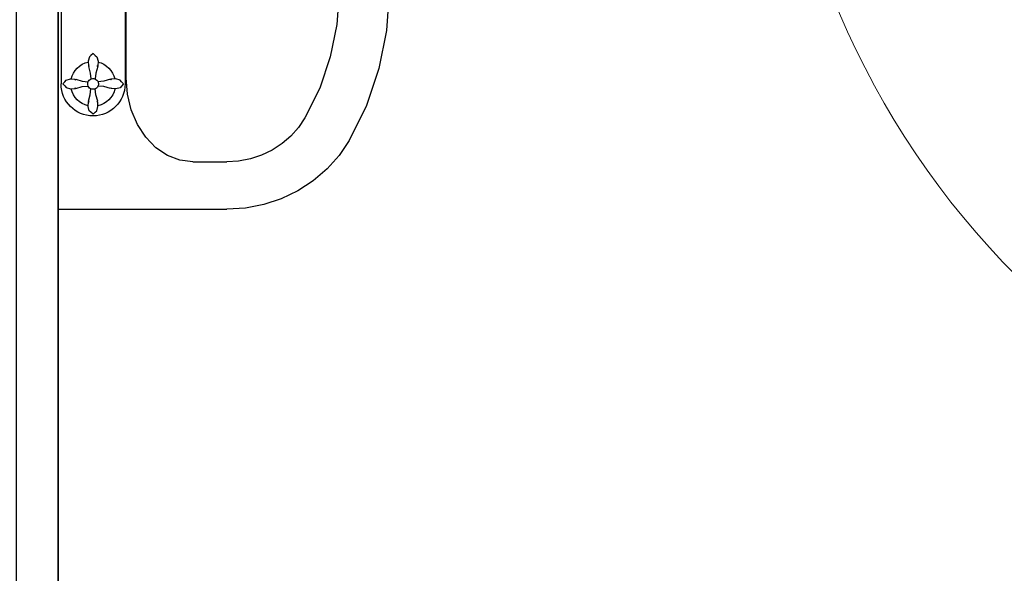
# Model space of a CAD drawing. Units: inches. Extents: x 3321 to 5237, y 11 to 1752.
# Tile 30 of 43: x 5060 to 5095, y 1396 to 1416. Entities that reach past the tile are written whole.
import ezdxf

# ---------------------------------------------------------------- set-up
doc = ezdxf.new("R2010")
doc.units = ezdxf.units.IN
for name, color, linetype, lineweight in [('A-ANNO-DIMS', 2, 'Continuous', 18), ('A-DOOR', 4, 'Continuous', 18), ('A-WALL', 7, 'Continuous', 35), ('Сантехника', 7, 'Continuous', 18)]:
    doc.layers.add(name, color=color, linetype=linetype, lineweight=lineweight)
doc.layers.add('SANTEH', color=7, linetype='Continuous')
doc.styles.get("Standard").update_dxf_attribs({"font": 'arial.ttf'})
doc.dimstyles.new('ISO-25', dxfattribs={"dimtxt": 9, "dimasz": 2.5, "dimexe": 1.25, "dimexo": 0.625, "dimtad": 1, "dimdec": 1, "dimlunit": 3, "dimtxsty": 'Standard', "dimcen": 2.5, "dimclrd": 4, "dimclre": 4, "dimclrt": 256, "dimadec": 0, "dimazin": 0, "dimtfac": 1, "dimtdec": 1, "dimtmove": 0, "dimatfit": 3, "dimfxl": 1, "dimarcsym": 0})

# ---------------------------------------------------------------- blocks, each defined once
blk = doc.blocks.new('*U8')
for p, q in [((-30, 0), (-30, 6)), ((0, 0), (0, 6))]:
    blk.add_line(p, q)
blk.add_lwpolyline([(0, 0), (0, -30), (-1.75, -30), (-1.75, 0)], close=True)
blk.add_arc((0, 0), 30, 180, 270)
blk = doc.blocks.new('Basin 01_71')
at = {"layer": 'SANTEH'}
for p, q in [((0, 350), (0, 171.8)), ((460, 350), (0, 350)), ((132.5, 345.3), (130.2, 343.2)), ((132.5, 345.3), (130.2, 343.2)), ((132.5, 345.3), (130.2, 343.2)), ((132.5, 345.3), (130.2, 343.2)), ((132.5, 345.3), (130.2, 343.2)), ((132.5, 345.3), (130.2, 343.2)), ((132.5, 346.9), (327.5, 346.9)), ((132.5, 345.3), (134.7, 343.2)), ((132.5, 345.3), (134.7, 343.2)), ((132.5, 345.3), (134.7, 343.2)), ((132.5, 345.3), (134.7, 343.2)), ((132.5, 345.3), (134.7, 343.2)), ((132.5, 345.3), (134.7, 343.2)), ((327.5, 345.3), (325.2, 343.2)), ((327.5, 345.3), (325.2, 343.2)), ((327.5, 345.3), (325.2, 343.2)), ((327.5, 345.3), (325.2, 343.2)), ((327.5, 345.3), (325.2, 343.2)), ((327.5, 345.3), (325.2, 343.2)), ((327.5, 345.3), (329.7, 343.2)), ((327.5, 345.3), (329.7, 343.2)), ((327.5, 345.3), (329.7, 343.2)), ((327.5, 345.3), (329.7, 343.2)), ((327.5, 345.3), (329.7, 343.2)), ((327.5, 345.3), (329.7, 343.2)), ((460, 350), (460, 171.8)), ((128.5, 341.7), (127.2, 337.2)), ((128.5, 341.7), (127.2, 337.2)), ((128.5, 341.7), (127.2, 337.2)), ((128.5, 341.7), (127.2, 337.2)), ((128.5, 341.7), (127.2, 337.2)), ((128.5, 341.7), (127.2, 337.2)), ((127.2, 337.2), (127.5, 332.3)), ((127.2, 337.2), (127.5, 332.3)), ((127.2, 337.2), (127.5, 332.3)), ((127.2, 337.2), (127.5, 332.3)), ((127.2, 337.2), (127.5, 332.3)), ((127.2, 337.2), (127.5, 332.3)), ((130.2, 343.2), (128.5, 341.7)), ((130.2, 343.2), (128.5, 341.7)), ((130.2, 343.2), (128.5, 341.7)), ((130.2, 343.2), (128.5, 341.7)), ((130.2, 343.2), (128.5, 341.7)), ((130.2, 343.2), (128.5, 341.7)), ((134.7, 343.2), (136.4, 341.7)), ((134.7, 343.2), (136.4, 341.7)), ((134.7, 343.2), (136.4, 341.7)), ((134.7, 343.2), (136.4, 341.7)), ((134.7, 343.2), (136.4, 341.7)), ((134.7, 343.2), (136.4, 341.7)), ((136.4, 341.7), (137.7, 337.2)), ((136.4, 341.7), (137.7, 337.2)), ((136.4, 341.7), (137.7, 337.2)), ((136.4, 341.7), (137.7, 337.2)), ((136.4, 341.7), (137.7, 337.2)), ((136.4, 341.7), (137.7, 337.2)), ((137.7, 337.2), (137.4, 332.3)), ((137.7, 337.2), (137.4, 332.3)), ((137.7, 337.2), (137.4, 332.3)), ((137.7, 337.2), (137.4, 332.3)), ((137.7, 337.2), (137.4, 332.3)), ((137.7, 337.2), (137.4, 332.3)), ((323.5, 341.7), (322.2, 337.2)), ((323.5, 341.7), (322.2, 337.2)), ((323.5, 341.7), (322.2, 337.2)), ((323.5, 341.7), (322.2, 337.2)), ((323.5, 341.7), (322.2, 337.2)), ((323.5, 341.7), (322.2, 337.2)), ((322.2, 337.2), (322.5, 332.3)), ((322.2, 337.2), (322.5, 332.3)), ((322.2, 337.2), (322.5, 332.3)), ((322.2, 337.2), (322.5, 332.3)), ((322.2, 337.2), (322.5, 332.3)), ((322.2, 337.2), (322.5, 332.3)), ((325.2, 343.2), (323.5, 341.7)), ((325.2, 343.2), (323.5, 341.7)), ((325.2, 343.2), (323.5, 341.7)), ((325.2, 343.2), (323.5, 341.7)), ((325.2, 343.2), (323.5, 341.7)), ((325.2, 343.2), (323.5, 341.7)), ((329.7, 343.2), (331.4, 341.7)), ((329.7, 343.2), (331.4, 341.7)), ((329.7, 343.2), (331.4, 341.7)), ((329.7, 343.2), (331.4, 341.7)), ((329.7, 343.2), (331.4, 341.7)), ((329.7, 343.2), (331.4, 341.7)), ((331.4, 341.7), (332.7, 337.2)), ((331.4, 341.7), (332.7, 337.2)), ((331.4, 341.7), (332.7, 337.2)), ((331.4, 341.7), (332.7, 337.2)), ((331.4, 341.7), (332.7, 337.2)), ((331.4, 341.7), (332.7, 337.2)), ((332.7, 337.2), (332.4, 332.3)), ((332.7, 337.2), (332.4, 332.3)), ((332.7, 337.2), (332.4, 332.3)), ((332.7, 337.2), (332.4, 332.3)), ((332.7, 337.2), (332.4, 332.3)), ((332.7, 337.2), (332.4, 332.3)), ((127.5, 332.3), (128.4, 332)), ((127.5, 332.3), (128.4, 332)), ((127.5, 332.3), (128.4, 332)), ((127.5, 332.3), (128.4, 332)), ((127.5, 332.3), (128.4, 332)), ((127.5, 332.3), (128.4, 332)), ((128.4, 332), (127.6, 331.5)), ((128.4, 332), (127.6, 331.5)), ((128.4, 332), (127.6, 331.5)), ((128.4, 332), (127.6, 331.5)), ((128.4, 332), (127.6, 331.5)), ((128.4, 332), (127.6, 331.5)), ((127.6, 331.5), (129.6, 324.7)), ((127.6, 331.5), (129.6, 324.7)), ((127.6, 331.5), (129.6, 324.7)), ((127.6, 331.5), (129.6, 324.7)), ((127.6, 331.5), (129.6, 324.7)), ((127.6, 331.5), (129.6, 324.7)), ((129.6, 324.7), (130.2, 318.4)), ((129.6, 324.7), (130.2, 318.4)), ((129.6, 324.7), (130.2, 318.4)), ((129.6, 324.7), (130.2, 318.4)), ((129.6, 324.7), (130.2, 318.4)), ((129.6, 324.7), (130.2, 318.4)), ((135.4, 324.7), (134.8, 318.4)), ((135.4, 324.7), (134.8, 318.4)), ((135.4, 324.7), (134.8, 318.4)), ((135.4, 324.7), (134.8, 318.4)), ((135.4, 324.7), (134.8, 318.4)), ((135.4, 324.7), (134.8, 318.4)), ((137.4, 331.5), (135.4, 324.7)), ((137.4, 331.5), (135.4, 324.7)), ((137.4, 331.5), (135.4, 324.7)), ((137.4, 331.5), (135.4, 324.7)), ((137.4, 331.5), (135.4, 324.7)), ((137.4, 331.5), (135.4, 324.7)), ((137.4, 332.3), (136.6, 332)), ((137.4, 332.3), (136.6, 332)), ((137.4, 332.3), (136.6, 332)), ((137.4, 332.3), (136.6, 332)), ((137.4, 332.3), (136.6, 332)), ((137.4, 332.3), (136.6, 332)), ((136.6, 332), (137.4, 331.5)), ((136.6, 332), (137.4, 331.5)), ((136.6, 332), (137.4, 331.5)), ((136.6, 332), (137.4, 331.5)), ((136.6, 332), (137.4, 331.5)), ((136.6, 332), (137.4, 331.5)), ((322.5, 332.3), (323.4, 332)), ((322.5, 332.3), (323.4, 332)), ((322.5, 332.3), (323.4, 332)), ((322.5, 332.3), (323.4, 332)), ((322.5, 332.3), (323.4, 332)), ((322.5, 332.3), (323.4, 332)), ((323.4, 332), (322.6, 331.5)), ((323.4, 332), (322.6, 331.5)), ((323.4, 332), (322.6, 331.5)), ((323.4, 332), (322.6, 331.5)), ((323.4, 332), (322.6, 331.5)), ((323.4, 332), (322.6, 331.5)), ((322.6, 331.5), (324.6, 324.7)), ((322.6, 331.5), (324.6, 324.7)), ((322.6, 331.5), (324.6, 324.7)), ((322.6, 331.5), (324.6, 324.7)), ((322.6, 331.5), (324.6, 324.7)), ((322.6, 331.5), (324.6, 324.7)), ((324.6, 324.7), (325.2, 318.4)), ((324.6, 324.7), (325.2, 318.4)), ((324.6, 324.7), (325.2, 318.4)), ((324.6, 324.7), (325.2, 318.4)), ((324.6, 324.7), (325.2, 318.4)), ((324.6, 324.7), (325.2, 318.4)), ((330.4, 324.7), (329.8, 318.4)), ((330.4, 324.7), (329.8, 318.4)), ((330.4, 324.7), (329.8, 318.4)), ((330.4, 324.7), (329.8, 318.4)), ((330.4, 324.7), (329.8, 318.4)), ((330.4, 324.7), (329.8, 318.4)), ((332.4, 331.5), (330.4, 324.7)), ((332.4, 331.5), (330.4, 324.7)), ((332.4, 331.5), (330.4, 324.7)), ((332.4, 331.5), (330.4, 324.7)), ((332.4, 331.5), (330.4, 324.7)), ((332.4, 331.5), (330.4, 324.7)), ((332.4, 332.3), (331.6, 332)), ((332.4, 332.3), (331.6, 332)), ((332.4, 332.3), (331.6, 332)), ((332.4, 332.3), (331.6, 332)), ((332.4, 332.3), (331.6, 332)), ((332.4, 332.3), (331.6, 332)), ((331.6, 332), (332.4, 331.5)), ((331.6, 332), (332.4, 331.5)), ((331.6, 332), (332.4, 331.5)), ((331.6, 332), (332.4, 331.5)), ((331.6, 332), (332.4, 331.5)), ((331.6, 332), (332.4, 331.5)), ((100.4, 313.2), (102.5, 315.4)), ((100.4, 313.2), (102.5, 315.4)), ((100.4, 313.2), (102.5, 315.4)), ((100.4, 313.2), (102.5, 315.4)), ((100.4, 313.2), (102.5, 315.4)), ((100.4, 313.2), (102.5, 315.4)), ((100.4, 313.2), (102.5, 310.9)), ((100.4, 313.2), (102.5, 310.9)), ((100.4, 313.2), (102.5, 310.9)), ((100.4, 313.2), (102.5, 310.9)), ((100.4, 313.2), (102.5, 310.9)), ((100.4, 313.2), (102.5, 310.9)), ((102.5, 315.4), (104, 317.1)), ((102.5, 315.4), (104, 317.1)), ((102.5, 315.4), (104, 317.1)), ((102.5, 315.4), (104, 317.1)), ((102.5, 315.4), (104, 317.1)), ((102.5, 315.4), (104, 317.1)), ((104, 317.1), (108.5, 318.4)), ((104, 317.1), (108.5, 318.4)), ((104, 317.1), (108.5, 318.4)), ((104, 317.1), (108.5, 318.4)), ((104, 317.1), (108.5, 318.4)), ((104, 317.1), (108.5, 318.4)), ((108.5, 318.4), (113.4, 318.1)), ((108.5, 318.4), (113.4, 318.1)), ((108.5, 318.4), (113.4, 318.1)), ((108.5, 318.4), (113.4, 318.1)), ((108.5, 318.4), (113.4, 318.1)), ((108.5, 318.4), (113.4, 318.1)), ((113.4, 318.1), (113.7, 317.3)), ((113.4, 318.1), (113.7, 317.3)), ((113.4, 318.1), (113.7, 317.3)), ((113.4, 318.1), (113.7, 317.3)), ((113.4, 318.1), (113.7, 317.3)), ((113.4, 318.1), (113.7, 317.3)), ((113.7, 317.3), (114.2, 318.1)), ((113.7, 317.3), (114.2, 318.1)), ((113.7, 317.3), (114.2, 318.1)), ((113.7, 317.3), (114.2, 318.1)), ((113.7, 317.3), (114.2, 318.1)), ((113.7, 317.3), (114.2, 318.1)), ((114.2, 318.1), (121, 316.1)), ((114.2, 318.1), (121, 316.1)), ((114.2, 318.1), (121, 316.1)), ((114.2, 318.1), (121, 316.1)), ((114.2, 318.1), (121, 316.1)), ((114.2, 318.1), (121, 316.1)), ((121, 316.1), (127.3, 315.5)), ((121, 316.1), (127.3, 315.5)), ((121, 316.1), (127.3, 315.5)), ((121, 316.1), (127.3, 315.5)), ((121, 316.1), (127.3, 315.5)), ((121, 316.1), (127.3, 315.5)), ((127.1, 315.1), (126.8, 313.9)), ((127.1, 315.1), (126.8, 313.9)), ((127.1, 315.1), (126.8, 313.9)), ((127.1, 315.1), (126.8, 313.9)), ((127.1, 315.1), (126.8, 313.9)), ((127.1, 315.1), (126.8, 313.9)), ((126.8, 313.9), (126.8, 312.5)), ((126.8, 313.9), (126.8, 312.5)), ((126.8, 313.9), (126.8, 312.5)), ((126.8, 313.9), (126.8, 312.5)), ((126.8, 313.9), (126.8, 312.5)), ((126.8, 313.9), (126.8, 312.5)), ((126.8, 312.5), (127.1, 311.2)), ((126.8, 312.5), (127.1, 311.2)), ((126.8, 312.5), (127.1, 311.2)), ((126.8, 312.5), (127.1, 311.2)), ((126.8, 312.5), (127.1, 311.2)), ((126.8, 312.5), (127.1, 311.2)), ((127.7, 316.3), (127.1, 315.1)), ((127.7, 316.3), (127.1, 315.1)), ((127.7, 316.3), (127.1, 315.1)), ((127.7, 316.3), (127.1, 315.1)), ((127.7, 316.3), (127.1, 315.1)), ((127.7, 316.3), (127.1, 315.1)), ((128.6, 317.3), (127.7, 316.3)), ((128.6, 317.3), (127.7, 316.3)), ((128.6, 317.3), (127.7, 316.3)), ((128.6, 317.3), (127.7, 316.3)), ((128.6, 317.3), (127.7, 316.3)), ((128.6, 317.3), (127.7, 316.3)), ((129.7, 318.1), (128.6, 317.3)), ((129.7, 318.1), (128.6, 317.3)), ((129.7, 318.1), (128.6, 317.3)), ((129.7, 318.1), (128.6, 317.3)), ((129.7, 318.1), (128.6, 317.3)), ((129.7, 318.1), (128.6, 317.3)), ((130.9, 318.7), (129.7, 318.1)), ((130.9, 318.7), (129.7, 318.1)), ((130.9, 318.7), (129.7, 318.1)), ((130.9, 318.7), (129.7, 318.1)), ((130.9, 318.7), (129.7, 318.1)), ((130.9, 318.7), (129.7, 318.1)), ((132.2, 318.9), (130.9, 318.7)), ((132.2, 318.9), (130.9, 318.7)), ((132.2, 318.9), (130.9, 318.7)), ((132.2, 318.9), (130.9, 318.7)), ((132.2, 318.9), (130.9, 318.7)), ((132.2, 318.9), (130.9, 318.7)), ((133.5, 318.8), (132.2, 318.9)), ((133.5, 318.8), (132.2, 318.9)), ((133.5, 318.8), (132.2, 318.9)), ((133.5, 318.8), (132.2, 318.9)), ((133.5, 318.8), (132.2, 318.9)), ((133.5, 318.8), (132.2, 318.9)), ((134.8, 318.4), (133.5, 318.8)), ((134.8, 318.4), (133.5, 318.8)), ((134.8, 318.4), (133.5, 318.8)), ((134.8, 318.4), (133.5, 318.8)), ((134.8, 318.4), (133.5, 318.8)), ((134.8, 318.4), (133.5, 318.8)), ((135.9, 317.8), (134.8, 318.4)), ((135.9, 317.8), (134.8, 318.4)), ((135.9, 317.8), (134.8, 318.4)), ((135.9, 317.8), (134.8, 318.4)), ((135.9, 317.8), (134.8, 318.4)), ((135.9, 317.8), (134.8, 318.4)), ((136.9, 316.9), (135.9, 317.8)), ((136.9, 316.9), (135.9, 317.8)), ((136.9, 316.9), (135.9, 317.8)), ((136.9, 316.9), (135.9, 317.8)), ((136.9, 316.9), (135.9, 317.8)), ((136.9, 316.9), (135.9, 317.8)), ((137.6, 315.8), (136.9, 316.9)), ((137.6, 315.8), (136.9, 316.9)), ((137.6, 315.8), (136.9, 316.9)), ((137.6, 315.8), (136.9, 316.9)), ((137.6, 315.8), (136.9, 316.9)), ((137.6, 315.8), (136.9, 316.9)), ((138, 314.5), (137.6, 315.8)), ((138, 314.5), (137.6, 315.8)), ((138, 314.5), (137.6, 315.8)), ((138, 314.5), (137.6, 315.8)), ((138, 314.5), (137.6, 315.8)), ((138, 314.5), (137.6, 315.8)), ((144, 316.1), (137.7, 315.5)), ((144, 316.1), (137.7, 315.5)), ((144, 316.1), (137.7, 315.5)), ((144, 316.1), (137.7, 315.5)), ((144, 316.1), (137.7, 315.5)), ((144, 316.1), (137.7, 315.5)), ((138.2, 313.2), (138, 314.5)), ((138.2, 313.2), (138, 314.5)), ((138.2, 313.2), (138, 314.5)), ((138.2, 313.2), (138, 314.5)), ((138.2, 313.2), (138, 314.5)), ((138.2, 313.2), (138, 314.5)), ((138, 311.9), (138.2, 313.2)), ((138, 311.9), (138.2, 313.2)), ((138, 311.9), (138.2, 313.2)), ((138, 311.9), (138.2, 313.2)), ((138, 311.9), (138.2, 313.2)), ((138, 311.9), (138.2, 313.2)), ((150.8, 318.1), (144, 316.1)), ((150.8, 318.1), (144, 316.1)), ((150.8, 318.1), (144, 316.1)), ((150.8, 318.1), (144, 316.1)), ((150.8, 318.1), (144, 316.1)), ((150.8, 318.1), (144, 316.1)), ((151.3, 317.3), (150.8, 318.1)), ((151.3, 317.3), (150.8, 318.1)), ((151.3, 317.3), (150.8, 318.1)), ((151.3, 317.3), (150.8, 318.1)), ((151.3, 317.3), (150.8, 318.1)), ((151.3, 317.3), (150.8, 318.1)), ((151.6, 318.1), (151.3, 317.3)), ((151.6, 318.1), (151.3, 317.3)), ((151.6, 318.1), (151.3, 317.3)), ((151.6, 318.1), (151.3, 317.3)), ((151.6, 318.1), (151.3, 317.3)), ((151.6, 318.1), (151.3, 317.3)), ((156.5, 318.4), (151.6, 318.1)), ((156.5, 318.4), (151.6, 318.1)), ((156.5, 318.4), (151.6, 318.1)), ((156.5, 318.4), (151.6, 318.1)), ((156.5, 318.4), (151.6, 318.1)), ((156.5, 318.4), (151.6, 318.1)), ((161, 317.2), (156.5, 318.4)), ((161, 317.2), (156.5, 318.4)), ((161, 317.2), (156.5, 318.4)), ((161, 317.2), (156.5, 318.4)), ((161, 317.2), (156.5, 318.4)), ((161, 317.2), (156.5, 318.4)), ((162.5, 315.4), (161, 317.2)), ((162.5, 315.4), (161, 317.2)), ((162.5, 315.4), (161, 317.2)), ((162.5, 315.4), (161, 317.2)), ((162.5, 315.4), (161, 317.2)), ((162.5, 315.4), (161, 317.2)), ((164.6, 313.2), (162.5, 315.4)), ((164.6, 313.2), (162.5, 315.4)), ((164.6, 313.2), (162.5, 315.4)), ((164.6, 313.2), (162.5, 315.4)), ((164.6, 313.2), (162.5, 315.4)), ((164.6, 313.2), (162.5, 315.4)), ((164.6, 313.2), (162.5, 311)), ((164.6, 313.2), (162.5, 311)), ((164.6, 313.2), (162.5, 311)), ((164.6, 313.2), (162.5, 311)), ((164.6, 313.2), (162.5, 311)), ((164.6, 313.2), (162.5, 311)), ((295.4, 313.2), (297.5, 315.4)), ((295.4, 313.2), (297.5, 315.4)), ((295.4, 313.2), (297.5, 315.4)), ((295.4, 313.2), (297.5, 315.4)), ((295.4, 313.2), (297.5, 315.4)), ((295.4, 313.2), (297.5, 315.4)), ((295.4, 313.2), (297.5, 310.9)), ((295.4, 313.2), (297.5, 310.9)), ((295.4, 313.2), (297.5, 310.9)), ((295.4, 313.2), (297.5, 310.9)), ((295.4, 313.2), (297.5, 310.9)), ((295.4, 313.2), (297.5, 310.9)), ((297.5, 315.4), (299, 317.1)), ((297.5, 315.4), (299, 317.1)), ((297.5, 315.4), (299, 317.1)), ((297.5, 315.4), (299, 317.1)), ((297.5, 315.4), (299, 317.1)), ((297.5, 315.4), (299, 317.1)), ((299, 317.1), (303.5, 318.4)), ((299, 317.1), (303.5, 318.4)), ((299, 317.1), (303.5, 318.4)), ((299, 317.1), (303.5, 318.4)), ((299, 317.1), (303.5, 318.4)), ((299, 317.1), (303.5, 318.4)), ((303.5, 318.4), (308.4, 318.1)), ((303.5, 318.4), (308.4, 318.1)), ((303.5, 318.4), (308.4, 318.1)), ((303.5, 318.4), (308.4, 318.1)), ((303.5, 318.4), (308.4, 318.1)), ((303.5, 318.4), (308.4, 318.1)), ((308.4, 318.1), (308.7, 317.3)), ((308.4, 318.1), (308.7, 317.3)), ((308.4, 318.1), (308.7, 317.3)), ((308.4, 318.1), (308.7, 317.3)), ((308.4, 318.1), (308.7, 317.3)), ((308.4, 318.1), (308.7, 317.3)), ((308.7, 317.3), (309.2, 318.1)), ((308.7, 317.3), (309.2, 318.1)), ((308.7, 317.3), (309.2, 318.1)), ((308.7, 317.3), (309.2, 318.1)), ((308.7, 317.3), (309.2, 318.1)), ((308.7, 317.3), (309.2, 318.1)), ((309.2, 318.1), (316, 316.1)), ((309.2, 318.1), (316, 316.1)), ((309.2, 318.1), (316, 316.1)), ((309.2, 318.1), (316, 316.1)), ((309.2, 318.1), (316, 316.1)), ((309.2, 318.1), (316, 316.1)), ((316, 316.1), (322.3, 315.5)), ((316, 316.1), (322.3, 315.5)), ((316, 316.1), (322.3, 315.5)), ((316, 316.1), (322.3, 315.5)), ((316, 316.1), (322.3, 315.5)), ((316, 316.1), (322.3, 315.5)), ((322.1, 315.1), (321.8, 313.9)), ((322.1, 315.1), (321.8, 313.9)), ((322.1, 315.1), (321.8, 313.9)), ((322.1, 315.1), (321.8, 313.9)), ((322.1, 315.1), (321.8, 313.9)), ((322.1, 315.1), (321.8, 313.9)), ((321.8, 313.9), (321.8, 312.5)), ((321.8, 313.9), (321.8, 312.5)), ((321.8, 313.9), (321.8, 312.5)), ((321.8, 313.9), (321.8, 312.5)), ((321.8, 313.9), (321.8, 312.5)), ((321.8, 313.9), (321.8, 312.5)), ((321.8, 312.5), (322.1, 311.2)), ((321.8, 312.5), (322.1, 311.2)), ((321.8, 312.5), (322.1, 311.2)), ((321.8, 312.5), (322.1, 311.2)), ((321.8, 312.5), (322.1, 311.2)), ((321.8, 312.5), (322.1, 311.2)), ((322.7, 316.3), (322.1, 315.1)), ((322.7, 316.3), (322.1, 315.1)), ((322.7, 316.3), (322.1, 315.1)), ((322.7, 316.3), (322.1, 315.1)), ((322.7, 316.3), (322.1, 315.1)), ((322.7, 316.3), (322.1, 315.1)), ((323.6, 317.3), (322.7, 316.3)), ((323.6, 317.3), (322.7, 316.3)), ((323.6, 317.3), (322.7, 316.3)), ((323.6, 317.3), (322.7, 316.3)), ((323.6, 317.3), (322.7, 316.3)), ((323.6, 317.3), (322.7, 316.3)), ((324.7, 318.1), (323.6, 317.3)), ((324.7, 318.1), (323.6, 317.3)), ((324.7, 318.1), (323.6, 317.3)), ((324.7, 318.1), (323.6, 317.3)), ((324.7, 318.1), (323.6, 317.3)), ((324.7, 318.1), (323.6, 317.3)), ((325.9, 318.7), (324.7, 318.1)), ((325.9, 318.7), (324.7, 318.1)), ((325.9, 318.7), (324.7, 318.1)), ((325.9, 318.7), (324.7, 318.1)), ((325.9, 318.7), (324.7, 318.1)), ((325.9, 318.7), (324.7, 318.1)), ((327.2, 318.9), (325.9, 318.7)), ((327.2, 318.9), (325.9, 318.7)), ((327.2, 318.9), (325.9, 318.7)), ((327.2, 318.9), (325.9, 318.7)), ((327.2, 318.9), (325.9, 318.7)), ((327.2, 318.9), (325.9, 318.7)), ((328.5, 318.8), (327.2, 318.9)), ((328.5, 318.8), (327.2, 318.9)), ((328.5, 318.8), (327.2, 318.9)), ((328.5, 318.8), (327.2, 318.9)), ((328.5, 318.8), (327.2, 318.9)), ((328.5, 318.8), (327.2, 318.9)), ((329.8, 318.4), (328.5, 318.8)), ((329.8, 318.4), (328.5, 318.8)), ((329.8, 318.4), (328.5, 318.8)), ((329.8, 318.4), (328.5, 318.8)), ((329.8, 318.4), (328.5, 318.8)), ((329.8, 318.4), (328.5, 318.8)), ((330.9, 317.8), (329.8, 318.4)), ((330.9, 317.8), (329.8, 318.4)), ((330.9, 317.8), (329.8, 318.4)), ((330.9, 317.8), (329.8, 318.4)), ((330.9, 317.8), (329.8, 318.4)), ((330.9, 317.8), (329.8, 318.4)), ((331.9, 316.9), (330.9, 317.8)), ((331.9, 316.9), (330.9, 317.8)), ((331.9, 316.9), (330.9, 317.8)), ((331.9, 316.9), (330.9, 317.8)), ((331.9, 316.9), (330.9, 317.8)), ((331.9, 316.9), (330.9, 317.8)), ((332.6, 315.8), (331.9, 316.9)), ((332.6, 315.8), (331.9, 316.9)), ((332.6, 315.8), (331.9, 316.9)), ((332.6, 315.8), (331.9, 316.9)), ((332.6, 315.8), (331.9, 316.9)), ((332.6, 315.8), (331.9, 316.9)), ((333, 314.5), (332.6, 315.8)), ((333, 314.5), (332.6, 315.8)), ((333, 314.5), (332.6, 315.8)), ((333, 314.5), (332.6, 315.8)), ((333, 314.5), (332.6, 315.8)), ((333, 314.5), (332.6, 315.8)), ((339, 316.1), (332.7, 315.5)), ((339, 316.1), (332.7, 315.5)), ((339, 316.1), (332.7, 315.5)), ((339, 316.1), (332.7, 315.5)), ((339, 316.1), (332.7, 315.5)), ((339, 316.1), (332.7, 315.5)), ((333.2, 313.2), (333, 314.5)), ((333.2, 313.2), (333, 314.5)), ((333.2, 313.2), (333, 314.5)), ((333.2, 313.2), (333, 314.5)), ((333.2, 313.2), (333, 314.5)), ((333.2, 313.2), (333, 314.5)), ((333, 311.9), (333.2, 313.2)), ((333, 311.9), (333.2, 313.2)), ((333, 311.9), (333.2, 313.2)), ((333, 311.9), (333.2, 313.2)), ((333, 311.9), (333.2, 313.2)), ((333, 311.9), (333.2, 313.2)), ((345.8, 318.1), (339, 316.1)), ((345.8, 318.1), (339, 316.1)), ((345.8, 318.1), (339, 316.1)), ((345.8, 318.1), (339, 316.1)), ((345.8, 318.1), (339, 316.1)), ((345.8, 318.1), (339, 316.1)), ((346.3, 317.3), (345.8, 318.1)), ((346.3, 317.3), (345.8, 318.1)), ((346.3, 317.3), (345.8, 318.1)), ((346.3, 317.3), (345.8, 318.1)), ((346.3, 317.3), (345.8, 318.1)), ((346.3, 317.3), (345.8, 318.1)), ((346.6, 318.1), (346.3, 317.3)), ((346.6, 318.1), (346.3, 317.3)), ((346.6, 318.1), (346.3, 317.3)), ((346.6, 318.1), (346.3, 317.3)), ((346.6, 318.1), (346.3, 317.3)), ((346.6, 318.1), (346.3, 317.3)), ((351.5, 318.4), (346.6, 318.1)), ((351.5, 318.4), (346.6, 318.1)), ((351.5, 318.4), (346.6, 318.1)), ((351.5, 318.4), (346.6, 318.1)), ((351.5, 318.4), (346.6, 318.1)), ((351.5, 318.4), (346.6, 318.1)), ((356, 317.2), (351.5, 318.4)), ((356, 317.2), (351.5, 318.4)), ((356, 317.2), (351.5, 318.4)), ((356, 317.2), (351.5, 318.4)), ((356, 317.2), (351.5, 318.4)), ((356, 317.2), (351.5, 318.4)), ((357.5, 315.4), (356, 317.2)), ((357.5, 315.4), (356, 317.2)), ((357.5, 315.4), (356, 317.2)), ((357.5, 315.4), (356, 317.2)), ((357.5, 315.4), (356, 317.2)), ((357.5, 315.4), (356, 317.2)), ((359.6, 313.2), (357.5, 315.4)), ((359.6, 313.2), (357.5, 315.4)), ((359.6, 313.2), (357.5, 315.4)), ((359.6, 313.2), (357.5, 315.4)), ((359.6, 313.2), (357.5, 315.4)), ((359.6, 313.2), (357.5, 315.4)), ((359.6, 313.2), (357.5, 311)), ((359.6, 313.2), (357.5, 311)), ((359.6, 313.2), (357.5, 311)), ((359.6, 313.2), (357.5, 311)), ((359.6, 313.2), (357.5, 311)), ((359.6, 313.2), (357.5, 311)), ((102.5, 310.9), (104, 309.2)), ((102.5, 310.9), (104, 309.2)), ((102.5, 310.9), (104, 309.2)), ((102.5, 310.9), (104, 309.2)), ((102.5, 310.9), (104, 309.2)), ((102.5, 310.9), (104, 309.2)), ((104, 309.2), (108.5, 307.9)), ((104, 309.2), (108.5, 307.9)), ((104, 309.2), (108.5, 307.9)), ((104, 309.2), (108.5, 307.9)), ((104, 309.2), (108.5, 307.9)), ((104, 309.2), (108.5, 307.9)), ((108.5, 307.9), (113.4, 308.2)), ((108.5, 307.9), (113.4, 308.2)), ((108.5, 307.9), (113.4, 308.2)), ((108.5, 307.9), (113.4, 308.2)), ((108.5, 307.9), (113.4, 308.2)), ((108.5, 307.9), (113.4, 308.2)), ((113.4, 308.2), (113.7, 309.1)), ((113.4, 308.2), (113.7, 309.1)), ((113.4, 308.2), (113.7, 309.1)), ((113.4, 308.2), (113.7, 309.1)), ((113.4, 308.2), (113.7, 309.1)), ((113.4, 308.2), (113.7, 309.1)), ((113.7, 309.1), (114.2, 308.3)), ((113.7, 309.1), (114.2, 308.3)), ((113.7, 309.1), (114.2, 308.3)), ((113.7, 309.1), (114.2, 308.3)), ((113.7, 309.1), (114.2, 308.3)), ((113.7, 309.1), (114.2, 308.3)), ((114.2, 308.3), (121, 310.3)), ((114.2, 308.3), (121, 310.3)), ((114.2, 308.3), (121, 310.3)), ((114.2, 308.3), (121, 310.3)), ((114.2, 308.3), (121, 310.3)), ((114.2, 308.3), (121, 310.3)), ((121, 310.3), (127.3, 310.9)), ((121, 310.3), (127.3, 310.9)), ((121, 310.3), (127.3, 310.9)), ((121, 310.3), (127.3, 310.9)), ((121, 310.3), (127.3, 310.9)), ((121, 310.3), (127.3, 310.9)), ((127.1, 311.2), (127.7, 310.1)), ((127.1, 311.2), (127.7, 310.1)), ((127.1, 311.2), (127.7, 310.1)), ((127.1, 311.2), (127.7, 310.1)), ((127.1, 311.2), (127.7, 310.1)), ((127.1, 311.2), (127.7, 310.1)), ((127.7, 310.1), (128.6, 309.1)), ((127.7, 310.1), (128.6, 309.1)), ((127.7, 310.1), (128.6, 309.1)), ((127.7, 310.1), (128.6, 309.1)), ((127.7, 310.1), (128.6, 309.1)), ((127.7, 310.1), (128.6, 309.1)), ((128.6, 309.1), (129.7, 308.3)), ((128.6, 309.1), (129.7, 308.3)), ((128.6, 309.1), (129.7, 308.3)), ((128.6, 309.1), (129.7, 308.3)), ((128.6, 309.1), (129.7, 308.3)), ((128.6, 309.1), (129.7, 308.3)), ((129.6, 301.7), (130.2, 308)), ((129.6, 301.7), (130.2, 308)), ((129.6, 301.7), (130.2, 308)), ((129.6, 301.7), (130.2, 308)), ((129.6, 301.7), (130.2, 308)), ((129.6, 301.7), (130.2, 308)), ((129.7, 308.3), (130.9, 307.7)), ((129.7, 308.3), (130.9, 307.7)), ((129.7, 308.3), (130.9, 307.7)), ((129.7, 308.3), (130.9, 307.7)), ((129.7, 308.3), (130.9, 307.7)), ((129.7, 308.3), (130.9, 307.7)), ((130.9, 307.7), (132.2, 307.5)), ((130.9, 307.7), (132.2, 307.5)), ((130.9, 307.7), (132.2, 307.5)), ((130.9, 307.7), (132.2, 307.5)), ((130.9, 307.7), (132.2, 307.5)), ((130.9, 307.7), (132.2, 307.5)), ((132.2, 307.5), (133.5, 307.6)), ((132.2, 307.5), (133.5, 307.6)), ((132.2, 307.5), (133.5, 307.6)), ((132.2, 307.5), (133.5, 307.6)), ((132.2, 307.5), (133.5, 307.6)), ((132.2, 307.5), (133.5, 307.6)), ((133.5, 307.6), (134.8, 308)), ((133.5, 307.6), (134.8, 308)), ((133.5, 307.6), (134.8, 308)), ((133.5, 307.6), (134.8, 308)), ((133.5, 307.6), (134.8, 308)), ((133.5, 307.6), (134.8, 308)), ((134.8, 308), (135.9, 308.6)), ((134.8, 308), (135.9, 308.6)), ((134.8, 308), (135.9, 308.6)), ((134.8, 308), (135.9, 308.6)), ((134.8, 308), (135.9, 308.6)), ((134.8, 308), (135.9, 308.6)), ((135.4, 301.7), (134.8, 308)), ((135.4, 301.7), (134.8, 308)), ((135.4, 301.7), (134.8, 308)), ((135.4, 301.7), (134.8, 308)), ((135.4, 301.7), (134.8, 308)), ((135.4, 301.7), (134.8, 308)), ((135.9, 308.6), (136.9, 309.5)), ((135.9, 308.6), (136.9, 309.5)), ((135.9, 308.6), (136.9, 309.5)), ((135.9, 308.6), (136.9, 309.5)), ((135.9, 308.6), (136.9, 309.5)), ((135.9, 308.6), (136.9, 309.5)), ((136.9, 309.5), (137.6, 310.6)), ((136.9, 309.5), (137.6, 310.6)), ((136.9, 309.5), (137.6, 310.6)), ((136.9, 309.5), (137.6, 310.6)), ((136.9, 309.5), (137.6, 310.6)), ((136.9, 309.5), (137.6, 310.6)), ((137.6, 310.6), (138, 311.9)), ((137.6, 310.6), (138, 311.9)), ((137.6, 310.6), (138, 311.9)), ((137.6, 310.6), (138, 311.9)), ((137.6, 310.6), (138, 311.9)), ((137.6, 310.6), (138, 311.9)), ((144, 310.3), (137.7, 310.9)), ((144, 310.3), (137.7, 310.9)), ((144, 310.3), (137.7, 310.9)), ((144, 310.3), (137.7, 310.9)), ((144, 310.3), (137.7, 310.9)), ((144, 310.3), (137.7, 310.9)), ((150.8, 308.3), (144, 310.3)), ((150.8, 308.3), (144, 310.3)), ((150.8, 308.3), (144, 310.3)), ((150.8, 308.3), (144, 310.3)), ((150.8, 308.3), (144, 310.3)), ((150.8, 308.3), (144, 310.3)), ((151.3, 309.1), (150.8, 308.3)), ((151.3, 309.1), (150.8, 308.3)), ((151.3, 309.1), (150.8, 308.3)), ((151.3, 309.1), (150.8, 308.3)), ((151.3, 309.1), (150.8, 308.3)), ((151.3, 309.1), (150.8, 308.3)), ((151.6, 308.3), (151.3, 309.1)), ((151.6, 308.3), (151.3, 309.1)), ((151.6, 308.3), (151.3, 309.1)), ((151.6, 308.3), (151.3, 309.1)), ((151.6, 308.3), (151.3, 309.1)), ((151.6, 308.3), (151.3, 309.1)), ((156.5, 308), (151.6, 308.3)), ((156.5, 308), (151.6, 308.3)), ((156.5, 308), (151.6, 308.3)), ((156.5, 308), (151.6, 308.3)), ((156.5, 308), (151.6, 308.3)), ((156.5, 308), (151.6, 308.3)), ((161, 309.2), (156.5, 308)), ((161, 309.2), (156.5, 308)), ((161, 309.2), (156.5, 308)), ((161, 309.2), (156.5, 308)), ((161, 309.2), (156.5, 308)), ((161, 309.2), (156.5, 308)), ((162.5, 311), (161, 309.2)), ((162.5, 311), (161, 309.2)), ((162.5, 311), (161, 309.2)), ((162.5, 311), (161, 309.2)), ((162.5, 311), (161, 309.2)), ((162.5, 311), (161, 309.2)), ((213.9, 305.1), (215, 298)), ((246.1, 305.1), (245, 298)), ((297.5, 310.9), (299, 309.2)), ((297.5, 310.9), (299, 309.2)), ((297.5, 310.9), (299, 309.2)), ((297.5, 310.9), (299, 309.2)), ((297.5, 310.9), (299, 309.2)), ((297.5, 310.9), (299, 309.2)), ((299, 309.2), (303.5, 307.9)), ((299, 309.2), (303.5, 307.9)), ((299, 309.2), (303.5, 307.9)), ((299, 309.2), (303.5, 307.9)), ((299, 309.2), (303.5, 307.9)), ((299, 309.2), (303.5, 307.9)), ((303.5, 307.9), (308.4, 308.2)), ((303.5, 307.9), (308.4, 308.2)), ((303.5, 307.9), (308.4, 308.2)), ((303.5, 307.9), (308.4, 308.2)), ((303.5, 307.9), (308.4, 308.2)), ((303.5, 307.9), (308.4, 308.2)), ((308.4, 308.2), (308.7, 309.1)), ((308.4, 308.2), (308.7, 309.1)), ((308.4, 308.2), (308.7, 309.1)), ((308.4, 308.2), (308.7, 309.1)), ((308.4, 308.2), (308.7, 309.1)), ((308.4, 308.2), (308.7, 309.1)), ((308.7, 309.1), (309.2, 308.3)), ((308.7, 309.1), (309.2, 308.3)), ((308.7, 309.1), (309.2, 308.3)), ((308.7, 309.1), (309.2, 308.3)), ((308.7, 309.1), (309.2, 308.3)), ((308.7, 309.1), (309.2, 308.3)), ((309.2, 308.3), (316, 310.3)), ((309.2, 308.3), (316, 310.3)), ((309.2, 308.3), (316, 310.3)), ((309.2, 308.3), (316, 310.3)), ((309.2, 308.3), (316, 310.3)), ((309.2, 308.3), (316, 310.3)), ((316, 310.3), (322.3, 310.9)), ((316, 310.3), (322.3, 310.9)), ((316, 310.3), (322.3, 310.9)), ((316, 310.3), (322.3, 310.9)), ((316, 310.3), (322.3, 310.9)), ((316, 310.3), (322.3, 310.9)), ((322.1, 311.2), (322.7, 310.1)), ((322.1, 311.2), (322.7, 310.1)), ((322.1, 311.2), (322.7, 310.1)), ((322.1, 311.2), (322.7, 310.1)), ((322.1, 311.2), (322.7, 310.1)), ((322.1, 311.2), (322.7, 310.1)), ((322.7, 310.1), (323.6, 309.1)), ((322.7, 310.1), (323.6, 309.1)), ((322.7, 310.1), (323.6, 309.1)), ((322.7, 310.1), (323.6, 309.1)), ((322.7, 310.1), (323.6, 309.1)), ((322.7, 310.1), (323.6, 309.1)), ((323.6, 309.1), (324.7, 308.3)), ((323.6, 309.1), (324.7, 308.3)), ((323.6, 309.1), (324.7, 308.3)), ((323.6, 309.1), (324.7, 308.3)), ((323.6, 309.1), (324.7, 308.3)), ((323.6, 309.1), (324.7, 308.3)), ((324.6, 301.7), (325.2, 308)), ((324.6, 301.7), (325.2, 308)), ((324.6, 301.7), (325.2, 308)), ((324.6, 301.7), (325.2, 308)), ((324.6, 301.7), (325.2, 308)), ((324.6, 301.7), (325.2, 308)), ((324.7, 308.3), (325.9, 307.7)), ((324.7, 308.3), (325.9, 307.7)), ((324.7, 308.3), (325.9, 307.7)), ((324.7, 308.3), (325.9, 307.7)), ((324.7, 308.3), (325.9, 307.7)), ((324.7, 308.3), (325.9, 307.7)), ((325.9, 307.7), (327.2, 307.5)), ((325.9, 307.7), (327.2, 307.5)), ((325.9, 307.7), (327.2, 307.5)), ((325.9, 307.7), (327.2, 307.5)), ((325.9, 307.7), (327.2, 307.5)), ((325.9, 307.7), (327.2, 307.5)), ((327.2, 307.5), (328.5, 307.6)), ((327.2, 307.5), (328.5, 307.6)), ((327.2, 307.5), (328.5, 307.6)), ((327.2, 307.5), (328.5, 307.6)), ((327.2, 307.5), (328.5, 307.6)), ((327.2, 307.5), (328.5, 307.6)), ((328.5, 307.6), (329.8, 308)), ((328.5, 307.6), (329.8, 308)), ((328.5, 307.6), (329.8, 308)), ((328.5, 307.6), (329.8, 308)), ((328.5, 307.6), (329.8, 308)), ((328.5, 307.6), (329.8, 308)), ((329.8, 308), (330.9, 308.6)), ((329.8, 308), (330.9, 308.6)), ((329.8, 308), (330.9, 308.6)), ((329.8, 308), (330.9, 308.6)), ((329.8, 308), (330.9, 308.6)), ((329.8, 308), (330.9, 308.6)), ((330.4, 301.7), (329.8, 308)), ((330.4, 301.7), (329.8, 308)), ((330.4, 301.7), (329.8, 308)), ((330.4, 301.7), (329.8, 308)), ((330.4, 301.7), (329.8, 308)), ((330.4, 301.7), (329.8, 308)), ((330.9, 308.6), (331.9, 309.5)), ((330.9, 308.6), (331.9, 309.5)), ((330.9, 308.6), (331.9, 309.5)), ((330.9, 308.6), (331.9, 309.5)), ((330.9, 308.6), (331.9, 309.5)), ((330.9, 308.6), (331.9, 309.5)), ((331.9, 309.5), (332.6, 310.6)), ((331.9, 309.5), (332.6, 310.6)), ((331.9, 309.5), (332.6, 310.6)), ((331.9, 309.5), (332.6, 310.6)), ((331.9, 309.5), (332.6, 310.6)), ((331.9, 309.5), (332.6, 310.6)), ((332.6, 310.6), (333, 311.9)), ((332.6, 310.6), (333, 311.9)), ((332.6, 310.6), (333, 311.9)), ((332.6, 310.6), (333, 311.9)), ((332.6, 310.6), (333, 311.9)), ((332.6, 310.6), (333, 311.9)), ((339, 310.3), (332.7, 310.9)), ((339, 310.3), (332.7, 310.9)), ((339, 310.3), (332.7, 310.9)), ((339, 310.3), (332.7, 310.9)), ((339, 310.3), (332.7, 310.9)), ((339, 310.3), (332.7, 310.9)), ((345.8, 308.3), (339, 310.3)), ((345.8, 308.3), (339, 310.3)), ((345.8, 308.3), (339, 310.3)), ((345.8, 308.3), (339, 310.3)), ((345.8, 308.3), (339, 310.3)), ((345.8, 308.3), (339, 310.3)), ((346.3, 309.1), (345.8, 308.3)), ((346.3, 309.1), (345.8, 308.3)), ((346.3, 309.1), (345.8, 308.3)), ((346.3, 309.1), (345.8, 308.3)), ((346.3, 309.1), (345.8, 308.3)), ((346.3, 309.1), (345.8, 308.3)), ((346.6, 308.3), (346.3, 309.1)), ((346.6, 308.3), (346.3, 309.1)), ((346.6, 308.3), (346.3, 309.1)), ((346.6, 308.3), (346.3, 309.1)), ((346.6, 308.3), (346.3, 309.1)), ((346.6, 308.3), (346.3, 309.1)), ((351.5, 308), (346.6, 308.3)), ((351.5, 308), (346.6, 308.3)), ((351.5, 308), (346.6, 308.3)), ((351.5, 308), (346.6, 308.3)), ((351.5, 308), (346.6, 308.3)), ((351.5, 308), (346.6, 308.3)), ((356, 309.2), (351.5, 308)), ((356, 309.2), (351.5, 308)), ((356, 309.2), (351.5, 308)), ((356, 309.2), (351.5, 308)), ((356, 309.2), (351.5, 308)), ((356, 309.2), (351.5, 308)), ((357.5, 311), (356, 309.2)), ((357.5, 311), (356, 309.2)), ((357.5, 311), (356, 309.2)), ((357.5, 311), (356, 309.2)), ((357.5, 311), (356, 309.2)), ((357.5, 311), (356, 309.2)), ((127.3, 289.2), (127.6, 294.1)), ((127.3, 289.2), (127.6, 294.1)), ((127.3, 289.2), (127.6, 294.1)), ((127.3, 289.2), (127.6, 294.1)), ((127.3, 289.2), (127.6, 294.1)), ((127.3, 289.2), (127.6, 294.1)), ((127.6, 294.9), (129.6, 301.7)), ((127.6, 294.9), (129.6, 301.7)), ((127.6, 294.9), (129.6, 301.7)), ((127.6, 294.9), (129.6, 301.7)), ((127.6, 294.9), (129.6, 301.7)), ((127.6, 294.9), (129.6, 301.7)), ((128.4, 294.4), (127.6, 294.9)), ((128.4, 294.4), (127.6, 294.9)), ((128.4, 294.4), (127.6, 294.9)), ((128.4, 294.4), (127.6, 294.9)), ((128.4, 294.4), (127.6, 294.9)), ((128.4, 294.4), (127.6, 294.9)), ((127.6, 294.1), (128.4, 294.4)), ((127.6, 294.1), (128.4, 294.4)), ((127.6, 294.1), (128.4, 294.4)), ((127.6, 294.1), (128.4, 294.4)), ((127.6, 294.1), (128.4, 294.4)), ((127.6, 294.1), (128.4, 294.4)), ((137.4, 294.9), (135.4, 301.7)), ((137.4, 294.9), (135.4, 301.7)), ((137.4, 294.9), (135.4, 301.7)), ((137.4, 294.9), (135.4, 301.7)), ((137.4, 294.9), (135.4, 301.7)), ((137.4, 294.9), (135.4, 301.7)), ((136.6, 294.4), (137.4, 294.9)), ((136.6, 294.4), (137.4, 294.9)), ((136.6, 294.4), (137.4, 294.9)), ((136.6, 294.4), (137.4, 294.9)), ((136.6, 294.4), (137.4, 294.9)), ((136.6, 294.4), (137.4, 294.9)), ((137.5, 294.1), (136.6, 294.4)), ((137.5, 294.1), (136.6, 294.4)), ((137.5, 294.1), (136.6, 294.4)), ((137.5, 294.1), (136.6, 294.4)), ((137.5, 294.1), (136.6, 294.4)), ((137.5, 294.1), (136.6, 294.4)), ((137.8, 289.2), (137.5, 294.1)), ((137.8, 289.2), (137.5, 294.1)), ((137.8, 289.2), (137.5, 294.1)), ((137.8, 289.2), (137.5, 294.1)), ((137.8, 289.2), (137.5, 294.1)), ((137.8, 289.2), (137.5, 294.1)), ((215, 298), (216.2, 284.6)), ((245, 298), (243.8, 284.6)), ((322.3, 289.2), (322.6, 294.1)), ((322.3, 289.2), (322.6, 294.1)), ((322.3, 289.2), (322.6, 294.1)), ((322.3, 289.2), (322.6, 294.1)), ((322.3, 289.2), (322.6, 294.1)), ((322.3, 289.2), (322.6, 294.1)), ((322.6, 294.9), (324.6, 301.7)), ((322.6, 294.9), (324.6, 301.7)), ((322.6, 294.9), (324.6, 301.7)), ((322.6, 294.9), (324.6, 301.7)), ((322.6, 294.9), (324.6, 301.7)), ((322.6, 294.9), (324.6, 301.7)), ((323.4, 294.4), (322.6, 294.9)), ((323.4, 294.4), (322.6, 294.9)), ((323.4, 294.4), (322.6, 294.9)), ((323.4, 294.4), (322.6, 294.9)), ((323.4, 294.4), (322.6, 294.9)), ((323.4, 294.4), (322.6, 294.9)), ((322.6, 294.1), (323.4, 294.4)), ((322.6, 294.1), (323.4, 294.4)), ((322.6, 294.1), (323.4, 294.4)), ((322.6, 294.1), (323.4, 294.4)), ((322.6, 294.1), (323.4, 294.4)), ((322.6, 294.1), (323.4, 294.4)), ((332.4, 294.9), (330.4, 301.7)), ((332.4, 294.9), (330.4, 301.7)), ((332.4, 294.9), (330.4, 301.7)), ((332.4, 294.9), (330.4, 301.7)), ((332.4, 294.9), (330.4, 301.7)), ((332.4, 294.9), (330.4, 301.7)), ((331.6, 294.4), (332.4, 294.9)), ((331.6, 294.4), (332.4, 294.9)), ((331.6, 294.4), (332.4, 294.9)), ((331.6, 294.4), (332.4, 294.9)), ((331.6, 294.4), (332.4, 294.9)), ((331.6, 294.4), (332.4, 294.9)), ((332.5, 294.1), (331.6, 294.4)), ((332.5, 294.1), (331.6, 294.4)), ((332.5, 294.1), (331.6, 294.4)), ((332.5, 294.1), (331.6, 294.4)), ((332.5, 294.1), (331.6, 294.4)), ((332.5, 294.1), (331.6, 294.4)), ((332.8, 289.2), (332.5, 294.1)), ((332.8, 289.2), (332.5, 294.1)), ((332.8, 289.2), (332.5, 294.1)), ((332.8, 289.2), (332.5, 294.1)), ((332.8, 289.2), (332.5, 294.1)), ((332.8, 289.2), (332.5, 294.1)), ((128.6, 284.7), (127.3, 289.2)), ((128.6, 284.7), (127.3, 289.2)), ((128.6, 284.7), (127.3, 289.2)), ((128.6, 284.7), (127.3, 289.2)), ((128.6, 284.7), (127.3, 289.2)), ((128.6, 284.7), (127.3, 289.2)), ((130.3, 283.2), (128.6, 284.7)), ((130.3, 283.2), (128.6, 284.7)), ((130.3, 283.2), (128.6, 284.7)), ((130.3, 283.2), (128.6, 284.7)), ((130.3, 283.2), (128.6, 284.7)), ((130.3, 283.2), (128.6, 284.7)), ((132.5, 281.1), (130.3, 283.2)), ((132.5, 281.1), (130.3, 283.2)), ((132.5, 281.1), (130.3, 283.2)), ((132.5, 281.1), (130.3, 283.2)), ((132.5, 281.1), (130.3, 283.2)), ((132.5, 281.1), (130.3, 283.2)), ((132.5, 281.1), (134.8, 283.2)), ((132.5, 281.1), (134.8, 283.2)), ((132.5, 281.1), (134.8, 283.2)), ((132.5, 281.1), (134.8, 283.2)), ((132.5, 281.1), (134.8, 283.2)), ((132.5, 281.1), (134.8, 283.2)), ((134.8, 283.2), (136.5, 284.7)), ((134.8, 283.2), (136.5, 284.7)), ((134.8, 283.2), (136.5, 284.7)), ((134.8, 283.2), (136.5, 284.7)), ((134.8, 283.2), (136.5, 284.7)), ((134.8, 283.2), (136.5, 284.7)), ((136.5, 284.7), (137.8, 289.2)), ((136.5, 284.7), (137.8, 289.2)), ((136.5, 284.7), (137.8, 289.2)), ((136.5, 284.7), (137.8, 289.2)), ((136.5, 284.7), (137.8, 289.2)), ((136.5, 284.7), (137.8, 289.2)), ((216.2, 284.6), (217.3, 266.6)), ((243.8, 284.6), (242.7, 266.6)), ((323.6, 284.7), (322.3, 289.2)), ((323.6, 284.7), (322.3, 289.2)), ((323.6, 284.7), (322.3, 289.2)), ((323.6, 284.7), (322.3, 289.2)), ((323.6, 284.7), (322.3, 289.2)), ((323.6, 284.7), (322.3, 289.2)), ((325.3, 283.2), (323.6, 284.7)), ((325.3, 283.2), (323.6, 284.7)), ((325.3, 283.2), (323.6, 284.7)), ((325.3, 283.2), (323.6, 284.7)), ((325.3, 283.2), (323.6, 284.7)), ((325.3, 283.2), (323.6, 284.7)), ((327.5, 281.1), (325.3, 283.2)), ((327.5, 281.1), (325.3, 283.2)), ((327.5, 281.1), (325.3, 283.2)), ((327.5, 281.1), (325.3, 283.2)), ((327.5, 281.1), (325.3, 283.2)), ((327.5, 281.1), (325.3, 283.2)), ((327.5, 281.1), (329.8, 283.2)), ((327.5, 281.1), (329.8, 283.2)), ((327.5, 281.1), (329.8, 283.2)), ((327.5, 281.1), (329.8, 283.2)), ((327.5, 281.1), (329.8, 283.2)), ((327.5, 281.1), (329.8, 283.2)), ((329.8, 283.2), (331.5, 284.7)), ((329.8, 283.2), (331.5, 284.7)), ((329.8, 283.2), (331.5, 284.7)), ((329.8, 283.2), (331.5, 284.7)), ((329.8, 283.2), (331.5, 284.7)), ((329.8, 283.2), (331.5, 284.7)), ((331.5, 284.7), (332.8, 289.2)), ((331.5, 284.7), (332.8, 289.2)), ((331.5, 284.7), (332.8, 289.2)), ((331.5, 284.7), (332.8, 289.2)), ((331.5, 284.7), (332.8, 289.2)), ((331.5, 284.7), (332.8, 289.2)), ((132.5, 279.4), (216.5, 279.4)), ((138.9, 278.2), (138.9, 278.2)), ((321.1, 278.2), (138.9, 278.2)), ((243.5, 279.4), (327.5, 279.4)), ((217.3, 266.6), (218.3, 252.4)), ((242.7, 266.6), (241.7, 252.4)), ((218.3, 252.4), (219.3, 245.4)), ((241.7, 252.4), (240.7, 245.4)), ((219.3, 245.4), (219, 234.8)), ((240.7, 245.4), (241, 234.8)), ((219, 234.8), (218.8, 221.1)), ((241, 234.8), (241.2, 221.1)), ((218.8, 221.1), (218.6, 209.8)), ((241.2, 221.1), (241.4, 209.8)), ((218.6, 209.8), (218.4, 198.7)), ((241.4, 209.8), (241.6, 198.7)), ((50, 207.5), (50, 171.8)), ((217, 200.3), (216.2, 196.2)), ((217.1, 200.6), (217, 200.3)), ((218.5, 202.5), (217.1, 200.6)), ((242.9, 200.6), (241.5, 202.5)), ((242.9, 200.6), (243, 200.3)), ((243.8, 196.2), (243, 200.3)), ((410, 207.5), (410, 171.8)), ((216.2, 196.2), (217, 192.1)), ((217, 192.1), (217.1, 191.8)), ((217.1, 191.8), (219.5, 188.3)), ((219.5, 188.3), (223.2, 185.6)), ((236.8, 185.6), (240.5, 188.3)), ((240.5, 188.3), (242.9, 191.8)), ((243, 192.1), (242.9, 191.8)), ((243, 192.1), (243.8, 196.2)), ((223.2, 185.6), (227.6, 184.2)), ((227.6, 184.2), (227.7, 184.2)), ((227.7, 184.2), (232.3, 184.2)), ((232.4, 184.2), (232.3, 184.2)), ((232.4, 184.2), (236.8, 185.6))]:
    blk.add_line(p, q, dxfattribs=at)
for points in [[(138.9, 278.2), (121.6, 276.9), (104.9, 272.8), (89.5, 266.3), (76, 257.5), (65, 246.8), (56.8, 234.5), (51.7, 221.3), (50, 207.5)], [(410, 207.5), (408.3, 221.3), (403.2, 234.5), (395, 246.8), (384, 257.5), (370.5, 266.3), (355.1, 272.8), (338.4, 276.9), (321.1, 278.2)], [(0, 171.8), (1.2, 152.1), (5, 132.7), (11.1, 114.1), (19.5, 96.5), (30.1, 80.2), (42.7, 65.6), (56.9, 52.9), (72.7, 42.3)], [(50, 171.8), (50.8, 159.2), (53.2, 146.8), (57.1, 134.9), (62.5, 123.6), (69.3, 113.2), (77.3, 103.8), (86.4, 95.7), (96.5, 89)], [(363.5, 89), (373.6, 95.7), (382.7, 103.8), (390.7, 113.2), (397.5, 123.6), (402.9, 134.9), (406.8, 146.8), (409.2, 159.2), (410, 171.8)], [(387.3, 42.3), (403.1, 52.9), (417.3, 65.6), (429.9, 80.2), (440.5, 96.5), (448.9, 114.1), (455, 132.7), (458.8, 152.1), (460, 171.8)], [(96.5, 89), (128, 73.4), (161.1, 62.2), (195.3, 55.3), (230, 53), (264.7, 55.3), (298.9, 62.2), (332, 73.4), (363.5, 89)], [(72.7, 42.3), (109.8, 24), (148.8, 10.8), (189.1, 2.7), (230, 0), (270.9, 2.7), (311.2, 10.8), (350.2, 24), (387.3, 42.3)]]:
    blk.add_lwpolyline(points, dxfattribs=at)
blk.add_circle((230, 188.9), 17.5, dxfattribs=at)
for centre, radius, start, end in [((132.5, 313.2), 33.8, 90, 270), ((327.5, 313.2), 33.8, 270, 90), ((132.5, 313.2), 23.7, 102.6646, 167.4213), ((132.5, 313.2), 23.7, 12.6646, 77.4213), ((327.5, 313.2), 23.7, 102.5787, 167.3354), ((327.5, 313.2), 23.7, 12.5787, 77.3354), ((230, 313.2), 18, 333.1469, 206.8531), ((132.5, 313.2), 23.7, 192.6646, 257.4213), ((132.5, 313.2), 23.7, 282.6646, 347.4213), ((327.5, 313.2), 23.7, 192.5787, 257.3354), ((327.5, 313.2), 23.7, 282.5787, 347.3354)]:
    blk.add_arc(centre, radius, start, end, dxfattribs=at)
blk = doc.blocks.new('*D197')
at = {"layer": 'A-ANNO-DIMS', "color": 4, "lineweight": -2, "transparency": 16777216}
for p, q in [((5117.009, 1364.83), (5117.009, 1476.212)), ((5114.11, 1364.83), (5118.259, 1364.83)), ((5117.009, 1343.839), (5117.009, 1362.33)), ((5114.11, 1341.339), (5118.259, 1341.339))]:
    blk.add_line(p, q, dxfattribs=at)
at = {"layer": 'A-ANNO-DIMS', "color": 4, "transparency": 16777216}
for points in [[(5116.592, 1362.33), (5117.426, 1362.33), (5117.009, 1364.83)], [(5116.592, 1343.839), (5117.426, 1343.839), (5117.009, 1341.339)]]:
    blk.add_solid(points, dxfattribs=at)
at = {"layer": 'Defpoints', "color": 0, "transparency": 16777216}
for p in [(5113.485, 1364.83), (5117.009, 1364.83), (5113.485, 1341.339)]:
    blk.add_point(p, dxfattribs=at)
at = {"layer": 'A-ANNO-DIMS', "transparency": 16777216, "insert": (5111.731, 1421.771), "char_height": 9, "attachment_point": 5, "rotation": 90}
blk.add_mtext('WC 1\'-11 1/2" TYP.', dxfattribs=at)
blk = doc.blocks.new('*D199')
at = {"layer": 'A-ANNO-DIMS', "color": 4, "lineweight": -2, "transparency": 16777216}
for p, q in [((5059.569, 1379.636), (5059.569, 1473.411)), ((5060.444, 1379.636), (5058.319, 1379.636)), ((5059.569, 1372.136), (5059.569, 1377.136)), ((5060.444, 1369.636), (5058.319, 1369.636))]:
    blk.add_line(p, q, dxfattribs=at)
at = {"layer": 'A-ANNO-DIMS', "color": 4, "transparency": 16777216}
for points in [[(5059.153, 1377.136), (5059.986, 1377.136), (5059.569, 1379.636)], [(5059.153, 1372.136), (5059.986, 1372.136), (5059.569, 1369.636)]]:
    blk.add_solid(points, dxfattribs=at)
at = {"layer": 'Defpoints', "color": 0, "transparency": 16777216}
for p in [(5059.569, 1379.636), (5061.069, 1379.636), (5061.069, 1369.636)]:
    blk.add_point(p, dxfattribs=at)
at = {"layer": 'A-ANNO-DIMS', "transparency": 16777216, "insert": (5054.349, 1427.773), "char_height": 9, "attachment_point": 5, "rotation": 90}
blk.add_mtext('TAP 0\'-10" TYP.', dxfattribs=at)

msp = doc.modelspace()

# ---------------------------------------------------------------- linework, layer by layer
at = {"layer": 'A-WALL'}
msp.add_line((5061.084, 1425.339), (5061.084, 1341.339), dxfattribs=at)

# ---------------------------------------------------------------- block references
at = {"layer": 'A-DOOR'}
msp.add_blockref('*U8', (5117.084, 1428.339), dxfattribs=at)
at = {"layer": 'Сантехника', "xscale": -0.0343047947041041, "yscale": 0.0343047947041041, "zscale": 0.0343047947041041, "rotation": 90}
msp.add_blockref('Basin 01_71', (5073.091, 1425.339), dxfattribs=at)

# ---------------------------------------------------------------- dimensions: what is measured, and where the dimension line sits
at = {"layer": 'A-ANNO-DIMS'}
for base, p1, p2, text, picture, middle in [((5117.009, 1364.83), (5113.485, 1341.339), (5113.485, 1364.83), 'WC <> TYP.', '*D197', (5111.731, 1421.771)), ((5059.569, 1379.636), (5061.069, 1369.636), (5061.069, 1379.636), 'TAP <> TYP.', '*D199', (5054.349, 1427.773))]:
    dim = msp.add_linear_dim(base=base, p1=p1, p2=p2, angle=90, text=text, dimstyle='ISO-25', override={"dimdec": 1, "dimlfac": 1, "dimrnd": 0, "dimzin": 1, "dimdsep": 46, "dimlunit": 4, "dimfrac": 2}, dxfattribs=at)
    dim.commit()
    dim.dimension.update_dxf_attribs({"geometry": picture, "text_midpoint": middle})

doc.saveas('drawing.dxf')
